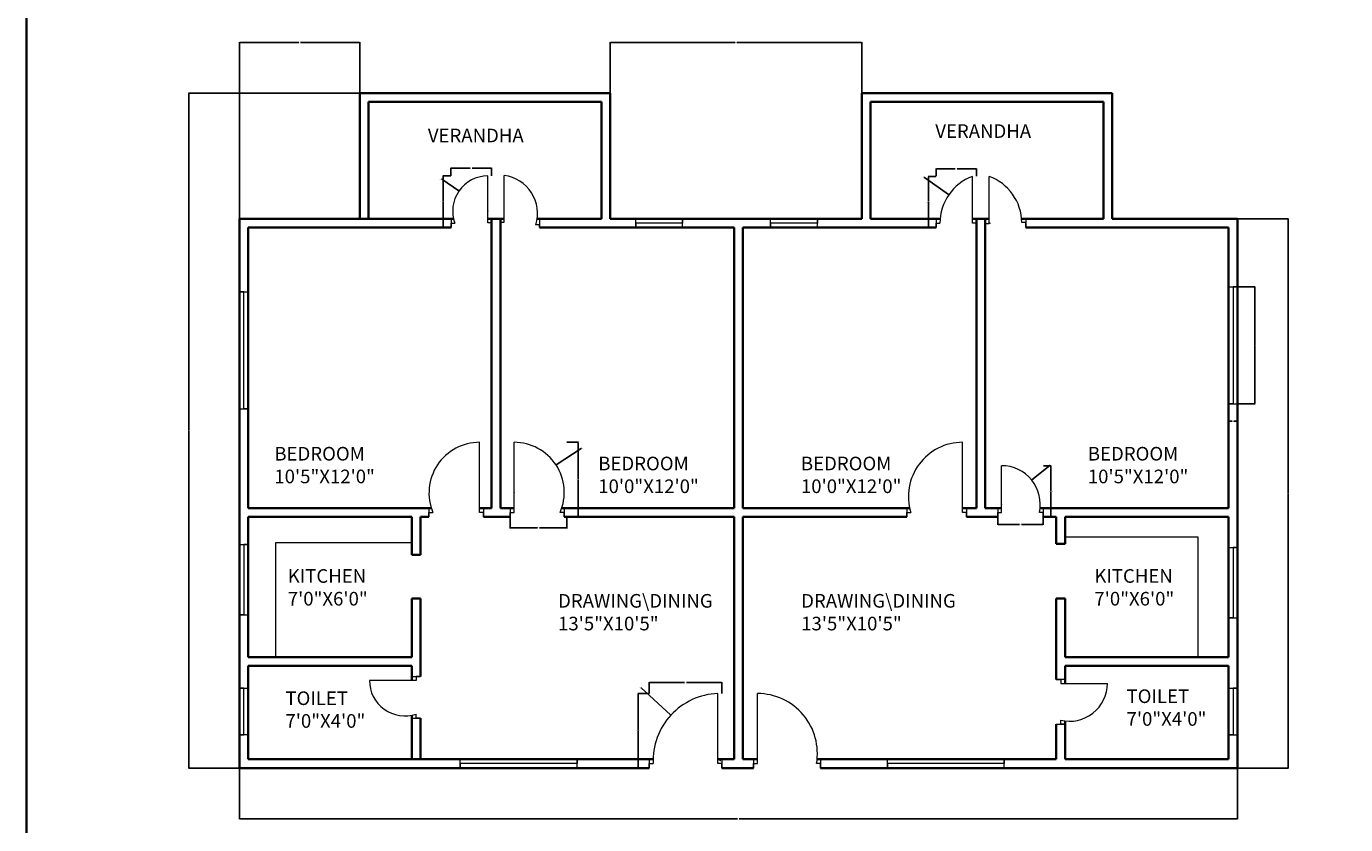
# Model space of a CAD drawing. Units: inches. Extents: x 2055 to 3558, y 1520 to 2888.
# Tile 3 of 8: x 2055 to 2732, y 2079 to 2489. Entities that reach past the tile are written whole.
import ezdxf

# ---------------------------------------------------------------- set-up
doc = ezdxf.new("R2010")
doc.units = ezdxf.units.IN
for name, color, linetype, lineweight in [('A-ANNO-DIMS', 2, 'Continuous', 18), ('A-ANNO-TTLB', 7, 'Continuous', 35), ('A-AREA-IDEN', 7, 'Continuous', 18), ('A-DOOR', 3, 'Continuous', 18), ('A-FLOR-FIXT', 8, 'Continuous', 18), ('A-GLAZ', 4, 'Continuous', 18), ('A-WALL', 7, 'Continuous', 35)]:
    doc.layers.add(name, color=color, linetype=linetype, lineweight=lineweight)
doc.styles.get("Standard").update_dxf_attribs({"font": 'arial.ttf'})
doc.dimstyles.get("Standard").update_dxf_attribs({"dimtxt": 0.18, "dimasz": 0.18, "dimexe": 0.18, "dimexo": 0.0625, "dimgap": 0.09, "dimtad": 0, "dimtih": 1, "dimtoh": 1, "dimdec": 4, "dimzin": 0, "dimdsep": 46, "dimtxsty": 'Standard', "dimcen": 0.09, "dimadec": 0, "dimazin": 0, "dimtfac": 1, "dimtdec": 4, "dimtofl": 0, "dimtmove": 0, "dimatfit": 3, "dimfxl": 1, "dimtolj": 1, "dimtzin": 0, "dimarcsym": 0})

# ---------------------------------------------------------------- blocks, each defined once
blk = doc.blocks.new('DOOR-BED-36-A')
for p, q in [((26, 2.25), (26, 38.25)), ((0, 4.5), (0, 0)), ((0, 0), (0, 2.25)), ((0, 2.25), (2, 2.25)), ((28, 2.25), (26, 2.25)), ((28, 4.5), (28, 0)), ((28, 0), (28, 2.25))]:
    blk.add_line(p, q)
blk.add_arc((26, 12.25), 26, 90, 202.62954)
blk = doc.blocks.new('DOOR-BED-36-B')
for p, q in [((2, 2.25), (2, 38.25)), ((0, 4.5), (0, 0)), ((0, 0), (0, 2.25)), ((0, 2.25), (2, 2.25)), ((27.66, 2.25), (25.66, 2.25)), ((27.66, 4.5), (27.66, 0)), ((27.66, 0), (27.66, 2.25))]:
    blk.add_line(p, q)
blk.add_arc((2, 12.47), 25.78, 336.6346, 90)
blk = doc.blocks.new('DOOR-BED-36-C')
for p, q in [((28.6, 2.25), (28.6, 38.25)), ((0, 4.5), (0, 0)), ((0, 0), (0, 2.25)), ((0, 2.25), (2, 2.25)), ((30.6, 2.25), (28.6, 2.25)), ((30.6, 4.5), (30.6, 0)), ((30.6, 0), (30.6, 2.25))]:
    blk.add_line(p, q)
blk.add_arc((28.6, 10.43), 27.83, 90, 197.08497)
blk = doc.blocks.new('DOOR-BED-24-A')
for p, q in [((2, 2.25), (2, 26.25)), ((0, 4.5), (0, 0)), ((0, 0), (0, 2.25)), ((0, 2.25), (2, 2.25)), ((23.39, 2.25), (21.39, 2.25)), ((23.39, 4.5), (23.39, 0)), ((23.39, 0), (23.39, 2.25))]:
    blk.add_line(p, q)
blk.add_arc((2, 6.42), 19.83, 347.8769, 90)
blk = doc.blocks.new('DOOR-BATH-24-A')
for p, q in [((4.5, 22.87), (0, 22.87)), ((0, 22.87), (2.25, 22.87)), ((2.25, 22.87), (2.25, 20.87)), ((2.25, 20.87), (26.25, 20.87)), ((2.25, 0), (2.25, 2)), ((0, 0), (4.5, 0)), ((4.5, 0), (2.25, 0))]:
    blk.add_line(p, q)
blk.add_arc((6.83, 20.87), 19.42, 256.35438, 0)
blk = doc.blocks.new('DOOR-ENTRY-36-A')
for p, q in [((2, 2.25), (2, 38.25)), ((0, 4.5), (0, 0)), ((0, 0), (0, 2.25)), ((0, 2.25), (2, 2.25)), ((34.35, 2.25), (32.35, 2.25)), ((34.35, 4.5), (34.35, 0)), ((34.35, 0), (34.35, 2.25))]:
    blk.add_line(p, q)
blk.add_arc((2, 7.46), 30.8, 350.26968, 90)
blk = doc.blocks.new('DOOR-ENTRY-36-B')
for p, q in [((35.2, 2.25), (35.2, 38.25)), ((0, 4.5), (0, 0)), ((0, 0), (0, 2.25)), ((0, 2.25), (2, 2.25)), ((37.2, 2.25), (35.2, 2.25)), ((37.2, 4.5), (37.2, 0)), ((37.2, 0), (37.2, 2.25))]:
    blk.add_line(p, q)
blk.add_arc((36.42, 3.82), 34.45, 92.03168, 182.60616)
blk = doc.blocks.new('DOOR-VERANDA-24-E')
for p, q in [((2, 2.71), (2, 26.71)), ((0, 2.71), (2, 2.71)), ((20.12, 1.44), (18.12, 1.44)), ((20.12, 4.5), (20.12, 0)), ((20.12, 0), (20.12, 1.44))]:
    blk.add_line(p, q)
blk.add_arc((-0.34, 7.44), 19.42, 342.01317, 83.06507)
blk = doc.blocks.new('DOOR-VERANDA-24-F')
for p, q in [((18.85, 2.51), (18.85, 26.51)), ((0, 4.5), (0, 0)), ((0, 0), (0, 2.25)), ((0, 2.25), (2, 2.25)), ((20.85, 2.51), (18.85, 2.51))]:
    blk.add_line(p, q)
blk.add_arc((18.85, 8.53), 17.98, 90, 200.4386)
blk = doc.blocks.new('DOOR-VERANDA-24-G')
for p, q in [((18.74, 2.29), (18.74, 26.29)), ((0, 4.5), (0, 0)), ((0, 0), (0, 2.25)), ((0, 2.25), (2, 2.25)), ((20.74, 2.29), (18.74, 2.29))]:
    blk.add_line(p, q)
blk.add_arc((27.63, 2.25), 25.63, 110.29699, 180)
blk = doc.blocks.new('DOOR-VERANDA-24-H')
for p, q in [((2, 2.19), (2, 26.19)), ((0, 2.19), (2, 2.19)), ((20.78, 2.69), (18.78, 2.69)), ((20.78, 4.5), (20.78, 0)), ((20.78, 0), (20.78, 2.69))]:
    blk.add_line(p, q)
blk.add_arc((-6.63, 2.38), 25.41, 0.68308, 70.14714)
blk = doc.blocks.new('DOOR-BATH-24-D')
for p, q in [((21.75, 21.33), (26.25, 21.33)), ((26.25, 21.33), (24, 21.33)), ((24, 21.33), (24, 19.33)), ((24, 19.33), (0, 19.33)), ((21.75, 0), (26.25, 0)), ((24, 0), (24, 2)), ((26.25, 0), (24, 0))]:
    blk.add_line(p, q)
blk.add_arc((18.26, 19.33), 18.26, 180, 288.33755)
blk = doc.blocks.new('WIN-36')
for p, q in [((2.25, 36), (0, 36)), ((0, 36), (4.5, 36)), ((2.25, 0), (2.25, 36)), ((0, 0), (4.5, 0)), ((4.5, 0), (2.25, 0))]:
    blk.add_line(p, q)
blk = doc.blocks.new('WIN-24')
for p, q in [((0, 24), (4.5, 24)), ((4.5, 24), (2.25, 24)), ((2.25, 24), (2.25, 0)), ((2.25, 0), (0, 0)), ((0, 0), (4.5, 0))]:
    blk.add_line(p, q)
blk = doc.blocks.new('WIN-24-2')
for p, q in [((2.25, 24), (0, 24)), ((0, 24), (4.5, 24)), ((2.25, 0), (2.25, 24)), ((4.5, 0), (0, 0)), ((0, 0), (2.25, 0))]:
    blk.add_line(p, q)
blk = doc.blocks.new('WIN-60')
for p, q in [((0, 60), (4.5, 60)), ((4.5, 60), (2.25, 60)), ((2.25, 60), (2.25, 0)), ((2.25, 0), (0, 0)), ((0, 0), (4.5, 0))]:
    blk.add_line(p, q)
blk = doc.blocks.new('COUNTER-1')
for p, q in [((70.02, 58.69), (0, 58.69)), ((0, 58.69), (0, 0))]:
    blk.add_line(p, q)
blk = doc.blocks.new('COUNTER-2')
for p, q in [((0, 61.79), (68.13, 61.79)), ((68.13, 61.79), (68.13, 0))]:
    blk.add_line(p, q)
blk = doc.blocks.new('VERANDA-PERIMETER')
for p, q in [((0, 0), (0, 64.5)), ((4.5, 64.5), (4.5, 4.5)), ((124.15, 4.5), (124.15, 64.5)), ((128.65, 64.5), (128.65, 4.5)), ((4.5, 0), (0, 0)), ((4.5, 4.5), (124.15, 4.5)), ((128.65, 0), (4.5, 0)), ((128.65, 4.5), (128.65, 0))]:
    blk.add_line(p, q)
blk = doc.blocks.new('*D44')
at = {"layer": 'A-ANNO-DIMS', "color": 0, "lineweight": -2, "transparency": 16777216}
for p, q in [((2676.74, 2355.07), (2685.85, 2355.07)), ((2685.67, 2354.89), (2685.67, 2325.25)), ((2685.67, 2295.25), (2685.67, 2324.88)), ((2676.74, 2295.07), (2685.85, 2295.07))]:
    blk.add_line(p, q, dxfattribs=at)
at = {"layer": 'A-ANNO-DIMS', "color": 0, "transparency": 16777216}
for points in [[(2685.64, 2354.89), (2685.7, 2354.89), (2685.67, 2355.07)], [(2685.64, 2295.25), (2685.7, 2295.25), (2685.67, 2295.07)]]:
    blk.add_solid(points, dxfattribs=at)
at = {"layer": 'Defpoints', "color": 0, "transparency": 16777216}
for p in [(2676.67, 2355.07), (2685.67, 2355.07), (2676.67, 2295.07)]:
    blk.add_point(p, dxfattribs=at)
at = {"layer": 'A-ANNO-DIMS', "color": 0, "transparency": 16777216, "insert": (2685.67, 2325.07), "char_height": 0.18, "attachment_point": 5}
blk.add_mtext('\\A1;WINDOW 60 TYP.', dxfattribs=at)
blk = doc.blocks.new('*D45')
at = {"layer": 'A-ANNO-DIMS', "color": 0, "lineweight": -2, "transparency": 16777216}
for p, q in [((2672.17, 2295), (2672.17, 2285.89)), ((2676.67, 2295), (2676.67, 2285.89)), ((2672.35, 2286.07), (2673.97, 2286.07)), ((2676.49, 2286.07), (2674.88, 2286.07))]:
    blk.add_line(p, q, dxfattribs=at)
at = {"layer": 'A-ANNO-DIMS', "color": 0, "transparency": 16777216}
for points in [[(2672.35, 2286.1), (2672.35, 2286.04), (2672.17, 2286.07)], [(2676.49, 2286.1), (2676.49, 2286.04), (2676.67, 2286.07)]]:
    blk.add_solid(points, dxfattribs=at)
at = {"layer": 'Defpoints', "color": 0, "transparency": 16777216}
for p in [(2672.17, 2295.07), (2676.67, 2295.07), (2676.67, 2286.07)]:
    blk.add_point(p, dxfattribs=at)
at = {"layer": 'A-ANNO-DIMS', "color": 0, "transparency": 16777216, "insert": (2674.42, 2286.07), "char_height": 0.18, "attachment_point": 5}
blk.add_mtext('\\A1;5 TYP.', dxfattribs=at)
blk = doc.blocks.new('*D54')
at = {"layer": 'A-ANNO-DIMS', "color": 0, "lineweight": -2, "transparency": 16777216}
for p, q in [((2332.38, 2275.25), (2338.24, 2275.25)), ((2338.06, 2275.07), (2338.06, 2256.31)), ((2338.06, 2237.18), (2338.06, 2255.94)), ((2332.38, 2237), (2338.24, 2237))]:
    blk.add_line(p, q, dxfattribs=at)
at = {"layer": 'A-ANNO-DIMS', "color": 0, "transparency": 16777216}
for points in [[(2338.03, 2275.07), (2338.09, 2275.07), (2338.06, 2275.25)], [(2338.03, 2237.18), (2338.09, 2237.18), (2338.06, 2237)]]:
    blk.add_solid(points, dxfattribs=at)
at = {"layer": 'Defpoints', "color": 0, "transparency": 16777216}
for p in [(2332.32, 2275.25), (2338.06, 2275.25), (2332.32, 2237)]:
    blk.add_point(p, dxfattribs=at)
at = {"layer": 'A-ANNO-DIMS', "color": 0, "transparency": 16777216, "insert": (2338.06, 2256.12), "char_height": 0.18, "attachment_point": 5}
blk.add_mtext('\\A1;BED DOOR 38 TYP.', dxfattribs=at)
blk = doc.blocks.new('*D55')
at = {"layer": 'A-ANNO-DIMS', "color": 0, "lineweight": -2, "transparency": 16777216}
for p, q in [((2303.21, 2236.94), (2303.21, 2231.08)), ((2332.32, 2236.94), (2332.32, 2231.08)), ((2303.39, 2231.26), (2317.24, 2231.26)), ((2332.14, 2231.26), (2318.3, 2231.26))]:
    blk.add_line(p, q, dxfattribs=at)
at = {"layer": 'A-ANNO-DIMS', "color": 0, "transparency": 16777216}
for points in [[(2303.39, 2231.29), (2303.39, 2231.23), (2303.21, 2231.26)], [(2332.14, 2231.29), (2332.14, 2231.23), (2332.32, 2231.26)]]:
    blk.add_solid(points, dxfattribs=at)
at = {"layer": 'Defpoints', "color": 0, "transparency": 16777216}
for p in [(2303.21, 2237), (2332.32, 2237), (2332.32, 2231.26)]:
    blk.add_point(p, dxfattribs=at)
at = {"layer": 'A-ANNO-DIMS', "color": 0, "transparency": 16777216, "insert": (2317.77, 2231.26), "char_height": 0.18, "attachment_point": 5}
blk.add_mtext('\\A1;29 TYP.', dxfattribs=at)
blk = doc.blocks.new('*D58')
at = {"layer": 'A-ANNO-DIMS', "color": 0, "lineweight": -2, "transparency": 16777216}
for p, q in [((2577.07, 2263.25), (2581.12, 2263.25)), ((2580.94, 2263.07), (2580.94, 2250.31)), ((2580.94, 2237.18), (2580.94, 2249.94)), ((2577.07, 2237), (2581.12, 2237))]:
    blk.add_line(p, q, dxfattribs=at)
at = {"layer": 'A-ANNO-DIMS', "color": 0, "transparency": 16777216}
for points in [[(2580.91, 2263.07), (2580.97, 2263.07), (2580.94, 2263.25)], [(2580.91, 2237.18), (2580.97, 2237.18), (2580.94, 2237)]]:
    blk.add_solid(points, dxfattribs=at)
at = {"layer": 'Defpoints', "color": 0, "transparency": 16777216}
for p in [(2577.01, 2263.25), (2580.94, 2263.25), (2577.01, 2237)]:
    blk.add_point(p, dxfattribs=at)
at = {"layer": 'A-ANNO-DIMS', "color": 0, "transparency": 16777216, "insert": (2580.94, 2250.12), "char_height": 0.18, "attachment_point": 5}
blk.add_mtext('\\A1;BED DOOR 26 TYP.', dxfattribs=at)
blk = doc.blocks.new('*D59')
at = {"layer": 'A-ANNO-DIMS', "color": 0, "lineweight": -2, "transparency": 16777216}
for p, q in [((2553.61, 2236.94), (2553.61, 2232.88)), ((2577.01, 2236.94), (2577.01, 2232.88)), ((2553.79, 2233.06), (2564.78, 2233.06)), ((2576.83, 2233.06), (2565.84, 2233.06))]:
    blk.add_line(p, q, dxfattribs=at)
at = {"layer": 'A-ANNO-DIMS', "color": 0, "transparency": 16777216}
for points in [[(2553.79, 2233.09), (2553.79, 2233.03), (2553.61, 2233.06)], [(2576.83, 2233.09), (2576.83, 2233.03), (2577.01, 2233.06)]]:
    blk.add_solid(points, dxfattribs=at)
at = {"layer": 'Defpoints', "color": 0, "transparency": 16777216}
for p in [(2553.61, 2237), (2577.01, 2237), (2577.01, 2233.06)]:
    blk.add_point(p, dxfattribs=at)
at = {"layer": 'A-ANNO-DIMS', "color": 0, "transparency": 16777216, "insert": (2565.31, 2233.06), "char_height": 0.18, "attachment_point": 5}
blk.add_mtext('\\A1;23 TYP.', dxfattribs=at)
blk = doc.blocks.new('*D64')
at = {"layer": 'A-ANNO-DIMS', "color": 0, "lineweight": -2, "transparency": 16777216}
for p, q in [((2374.6, 2146.25), (2368.74, 2146.25)), ((2368.92, 2146.07), (2368.92, 2127.31)), ((2368.92, 2108.18), (2368.92, 2126.94)), ((2374.6, 2108), (2368.74, 2108))]:
    blk.add_line(p, q, dxfattribs=at)
at = {"layer": 'A-ANNO-DIMS', "color": 0, "transparency": 16777216}
for points in [[(2368.89, 2146.07), (2368.95, 2146.07), (2368.92, 2146.25)], [(2368.89, 2108.18), (2368.95, 2108.18), (2368.92, 2108)]]:
    blk.add_solid(points, dxfattribs=at)
at = {"layer": 'Defpoints', "color": 0, "transparency": 16777216}
for p in [(2368.92, 2146.25), (2374.66, 2146.25), (2374.66, 2108)]:
    blk.add_point(p, dxfattribs=at)
at = {"layer": 'A-ANNO-DIMS', "color": 0, "transparency": 16777216, "insert": (2368.92, 2127.12), "char_height": 0.18, "attachment_point": 5}
blk.add_mtext('\\A1;ENTRY DOOR 38 TYP.', dxfattribs=at)
blk = doc.blocks.new('*D65')
at = {"layer": 'A-ANNO-DIMS', "color": 0, "lineweight": -2, "transparency": 16777216}
for p, q in [((2374.66, 2146.31), (2374.66, 2152.17)), ((2374.84, 2151.99), (2392.73, 2151.99)), ((2411.68, 2151.99), (2393.79, 2151.99)), ((2411.86, 2146.31), (2411.86, 2152.17))]:
    blk.add_line(p, q, dxfattribs=at)
at = {"layer": 'A-ANNO-DIMS', "color": 0, "transparency": 16777216}
for points in [[(2374.84, 2152.02), (2374.84, 2151.96), (2374.66, 2151.99)], [(2411.68, 2152.02), (2411.68, 2151.96), (2411.86, 2151.99)]]:
    blk.add_solid(points, dxfattribs=at)
at = {"layer": 'Defpoints', "color": 0, "transparency": 16777216}
for p in [(2411.86, 2151.99), (2374.66, 2146.25), (2411.86, 2146.25)]:
    blk.add_point(p, dxfattribs=at)
at = {"layer": 'A-ANNO-DIMS', "color": 0, "transparency": 16777216, "insert": (2393.26, 2151.99), "char_height": 0.18, "attachment_point": 5}
blk.add_mtext('\\A1;37 TYP.', dxfattribs=at)
blk = doc.blocks.new('*D92')
at = {"layer": 'A-ANNO-DIMS', "color": 0, "lineweight": -2, "transparency": 16777216}
for p, q in [((2272.7, 2412.01), (2268.61, 2412.01)), ((2268.79, 2411.83), (2268.79, 2398.94)), ((2268.79, 2385.68), (2268.79, 2398.57)), ((2272.7, 2385.5), (2268.61, 2385.5))]:
    blk.add_line(p, q, dxfattribs=at)
at = {"layer": 'A-ANNO-DIMS', "color": 0, "transparency": 16777216}
for points in [[(2268.76, 2411.83), (2268.82, 2411.83), (2268.79, 2412.01)], [(2268.76, 2385.68), (2268.82, 2385.68), (2268.79, 2385.5)]]:
    blk.add_solid(points, dxfattribs=at)
at = {"layer": 'Defpoints', "color": 0, "transparency": 16777216}
for p in [(2268.79, 2412.01), (2272.77, 2412.01), (2272.77, 2385.5)]:
    blk.add_point(p, dxfattribs=at)
at = {"layer": 'A-ANNO-DIMS', "color": 0, "transparency": 16777216, "insert": (2268.79, 2398.76), "char_height": 0.18, "attachment_point": 5}
blk.add_mtext('\\A1;VERANDA DOOR 27 TYP.', dxfattribs=at)
blk = doc.blocks.new('*D93')
at = {"layer": 'A-ANNO-DIMS', "color": 0, "lineweight": -2, "transparency": 16777216}
for p, q in [((2272.77, 2412.08), (2272.77, 2416.17)), ((2272.95, 2415.99), (2282.69, 2415.99)), ((2293.49, 2415.99), (2283.75, 2415.99)), ((2293.67, 2412.08), (2293.67, 2416.17))]:
    blk.add_line(p, q, dxfattribs=at)
at = {"layer": 'A-ANNO-DIMS', "color": 0, "transparency": 16777216}
for points in [[(2272.95, 2416.02), (2272.95, 2415.96), (2272.77, 2415.99)], [(2293.49, 2416.02), (2293.49, 2415.96), (2293.67, 2415.99)]]:
    blk.add_solid(points, dxfattribs=at)
at = {"layer": 'Defpoints', "color": 0, "transparency": 16777216}
for p in [(2272.77, 2412.01), (2293.67, 2415.99), (2293.67, 2412.01)]:
    blk.add_point(p, dxfattribs=at)
at = {"layer": 'A-ANNO-DIMS', "color": 0, "transparency": 16777216, "insert": (2283.22, 2415.99), "char_height": 0.18, "attachment_point": 5}
blk.add_mtext('\\A1;21 TYP.', dxfattribs=at)
blk = doc.blocks.new('*D94')
at = {"layer": 'A-ANNO-DIMS', "color": 0, "lineweight": -2, "transparency": 16777216}
for p, q in [((2521.87, 2411.79), (2517.81, 2411.79)), ((2517.99, 2411.61), (2517.99, 2398.83)), ((2517.99, 2385.68), (2517.99, 2398.46)), ((2521.87, 2385.5), (2517.81, 2385.5))]:
    blk.add_line(p, q, dxfattribs=at)
at = {"layer": 'A-ANNO-DIMS', "color": 0, "transparency": 16777216}
for points in [[(2517.96, 2411.61), (2518.02, 2411.61), (2517.99, 2411.79)], [(2517.96, 2385.68), (2518.02, 2385.68), (2517.99, 2385.5)]]:
    blk.add_solid(points, dxfattribs=at)
at = {"layer": 'Defpoints', "color": 0, "transparency": 16777216}
for p in [(2517.99, 2411.79), (2521.94, 2411.79), (2521.94, 2385.5)]:
    blk.add_point(p, dxfattribs=at)
at = {"layer": 'A-ANNO-DIMS', "color": 0, "transparency": 16777216, "insert": (2517.99, 2398.64), "char_height": 0.18, "attachment_point": 5}
blk.add_mtext('\\A1;VERANDA DOOR 26 TYP.', dxfattribs=at)
blk = doc.blocks.new('*D95')
at = {"layer": 'A-ANNO-DIMS', "color": 0, "lineweight": -2, "transparency": 16777216}
for p, q in [((2521.94, 2411.85), (2521.94, 2415.91)), ((2522.12, 2415.73), (2531.78, 2415.73)), ((2542.49, 2415.73), (2532.84, 2415.73)), ((2542.67, 2411.85), (2542.67, 2415.91))]:
    blk.add_line(p, q, dxfattribs=at)
at = {"layer": 'A-ANNO-DIMS', "color": 0, "transparency": 16777216}
for points in [[(2522.12, 2415.76), (2522.12, 2415.7), (2521.94, 2415.73)], [(2542.49, 2415.76), (2542.49, 2415.7), (2542.67, 2415.73)]]:
    blk.add_solid(points, dxfattribs=at)
at = {"layer": 'Defpoints', "color": 0, "transparency": 16777216}
for p in [(2542.67, 2415.73), (2521.94, 2411.79), (2542.67, 2411.79)]:
    blk.add_point(p, dxfattribs=at)
at = {"layer": 'A-ANNO-DIMS', "color": 0, "transparency": 16777216, "insert": (2532.31, 2415.73), "char_height": 0.18, "attachment_point": 5}
blk.add_mtext('\\A1;21 TYP.', dxfattribs=at)
blk = doc.blocks.new('*D118')
at = {"layer": 'A-ANNO-DIMS', "color": 0, "lineweight": -2, "transparency": 16777216}
for p, q in [((2164.17, 2107.94), (2164.17, 2081.77)), ((2676.67, 2107.94), (2676.67, 2081.77)), ((2164.35, 2081.95), (2420.03, 2081.95)), ((2676.49, 2081.95), (2420.82, 2081.95))]:
    blk.add_line(p, q, dxfattribs=at)
at = {"layer": 'A-ANNO-DIMS', "color": 0, "transparency": 16777216}
for points in [[(2164.35, 2081.98), (2164.35, 2081.92), (2164.17, 2081.95)], [(2676.49, 2081.98), (2676.49, 2081.92), (2676.67, 2081.95)]]:
    blk.add_solid(points, dxfattribs=at)
at = {"layer": 'Defpoints', "color": 0, "transparency": 16777216}
for p in [(2164.17, 2108), (2676.67, 2108), (2676.67, 2081.95)]:
    blk.add_point(p, dxfattribs=at)
at = {"layer": 'A-ANNO-DIMS', "color": 0, "transparency": 16777216, "insert": (2420.42, 2081.95), "char_height": 0.18, "attachment_point": 5}
blk.add_mtext('\\A1;512.5', dxfattribs=at)
blk = doc.blocks.new('*D119')
at = {"layer": 'A-ANNO-DIMS', "color": 0, "lineweight": -2, "transparency": 16777216}
for p, q in [((2225.88, 2454.5), (2137.94, 2454.5)), ((2138.12, 2454.32), (2138.12, 2281.43)), ((2138.12, 2108.18), (2138.12, 2281.07)), ((2164.11, 2108), (2137.94, 2108))]:
    blk.add_line(p, q, dxfattribs=at)
at = {"layer": 'A-ANNO-DIMS', "color": 0, "transparency": 16777216}
for points in [[(2138.09, 2454.32), (2138.15, 2454.32), (2138.12, 2454.5)], [(2138.09, 2108.18), (2138.15, 2108.18), (2138.12, 2108)]]:
    blk.add_solid(points, dxfattribs=at)
at = {"layer": 'Defpoints', "color": 0, "transparency": 16777216}
for p in [(2138.12, 2454.5), (2225.95, 2454.5), (2164.17, 2108)]:
    blk.add_point(p, dxfattribs=at)
at = {"layer": 'A-ANNO-DIMS', "color": 0, "transparency": 16777216, "insert": (2138.12, 2281.25), "char_height": 0.18, "attachment_point": 5}
blk.add_mtext('\\A1;346.5', dxfattribs=at)
blk = doc.blocks.new('*D120')
at = {"layer": 'A-ANNO-DIMS', "color": 0, "lineweight": -2, "transparency": 16777216}
for p, q in [((2676.74, 2390), (2702.9, 2390)), ((2702.72, 2389.82), (2702.72, 2249.18)), ((2702.72, 2108.18), (2702.72, 2248.82)), ((2676.74, 2108), (2702.9, 2108))]:
    blk.add_line(p, q, dxfattribs=at)
at = {"layer": 'A-ANNO-DIMS', "color": 0, "transparency": 16777216}
for points in [[(2702.69, 2389.82), (2702.75, 2389.82), (2702.72, 2390)], [(2702.69, 2108.18), (2702.75, 2108.18), (2702.72, 2108)]]:
    blk.add_solid(points, dxfattribs=at)
at = {"layer": 'Defpoints', "color": 0, "transparency": 16777216}
for p in [(2676.67, 2390), (2702.72, 2390), (2676.67, 2108)]:
    blk.add_point(p, dxfattribs=at)
at = {"layer": 'A-ANNO-DIMS', "color": 0, "transparency": 16777216, "insert": (2702.72, 2249), "char_height": 0.18, "attachment_point": 5}
blk.add_mtext('\\A1;282', dxfattribs=at)
blk = doc.blocks.new('*D126')
at = {"layer": 'A-ANNO-DIMS', "color": 0, "lineweight": -2, "transparency": 16777216}
for p, q in [((2164.17, 2390.06), (2164.17, 2480.73)), ((2164.35, 2480.55), (2194.67, 2480.55)), ((2225.77, 2480.55), (2195.45, 2480.55)), ((2225.95, 2390.06), (2225.95, 2480.73))]:
    blk.add_line(p, q, dxfattribs=at)
at = {"layer": 'A-ANNO-DIMS', "color": 0, "transparency": 16777216}
for points in [[(2164.35, 2480.58), (2164.35, 2480.52), (2164.17, 2480.55)], [(2225.77, 2480.58), (2225.77, 2480.52), (2225.95, 2480.55)]]:
    blk.add_solid(points, dxfattribs=at)
at = {"layer": 'Defpoints', "color": 0, "transparency": 16777216}
for p in [(2225.95, 2480.55), (2164.17, 2390), (2225.95, 2390)]:
    blk.add_point(p, dxfattribs=at)
at = {"layer": 'A-ANNO-DIMS', "color": 0, "transparency": 16777216, "insert": (2195.06, 2480.55), "char_height": 0.18, "attachment_point": 5}
blk.add_mtext('\\A1;61.77', dxfattribs=at)
blk = doc.blocks.new('*D127')
at = {"layer": 'A-ANNO-DIMS', "color": 0, "lineweight": -2, "transparency": 16777216}
for p, q in [((2354.59, 2454.56), (2354.59, 2480.73)), ((2354.77, 2480.55), (2418.72, 2480.55)), ((2483.58, 2480.55), (2419.63, 2480.55)), ((2483.76, 2454.56), (2483.76, 2480.73))]:
    blk.add_line(p, q, dxfattribs=at)
at = {"layer": 'A-ANNO-DIMS', "color": 0, "transparency": 16777216}
for points in [[(2354.77, 2480.58), (2354.77, 2480.52), (2354.59, 2480.55)], [(2483.58, 2480.58), (2483.58, 2480.52), (2483.76, 2480.55)]]:
    blk.add_solid(points, dxfattribs=at)
at = {"layer": 'Defpoints', "color": 0, "transparency": 16777216}
for p in [(2483.76, 2480.55), (2354.59, 2454.5), (2483.76, 2454.5)]:
    blk.add_point(p, dxfattribs=at)
at = {"layer": 'A-ANNO-DIMS', "color": 0, "transparency": 16777216, "insert": (2419.17, 2480.55), "char_height": 0.18, "attachment_point": 5}
blk.add_mtext('\\A1;129.16', dxfattribs=at)
blk = doc.blocks.new('*D161')
at = {"layer": 'A-ANNO-DIMS', "color": 0, "lineweight": -2, "transparency": 16777216}
for p, q in [((2370.37, 2149.19), (2370.55, 2149.19)), ((2370.55, 2149.19), (2385.62, 2135.3)), ((2410.99, 2111.82), (2411.17, 2111.82)), ((2411.08, 2111.73), (2411.08, 2111.91))]:
    blk.add_line(p, q, dxfattribs=at)
at = {"layer": 'A-ANNO-DIMS', "color": 0, "transparency": 16777216}
blk.add_solid([(2385.64, 2135.32), (2385.6, 2135.27), (2385.75, 2135.17)], dxfattribs=at)
at = {"layer": 'Defpoints', "color": 0, "transparency": 16777216}
for p in [(2385.75, 2135.17), (2411.08, 2111.82)]:
    blk.add_point(p, dxfattribs=at)
at = {"layer": 'A-ANNO-DIMS', "color": 0, "transparency": 16777216, "insert": (2369.82, 2149.19), "char_height": 0.18, "attachment_point": 5}
blk.add_mtext('\\A1;R34.455', dxfattribs=at)
blk = doc.blocks.new('*D165')
at = {"layer": 'A-ANNO-DIMS', "color": 0, "lineweight": -2, "transparency": 16777216}
for p, q in [((2339.68, 2272.13), (2326.9, 2263.73)), ((2339.86, 2272.13), (2339.68, 2272.13)), ((2305.12, 2249.47), (2305.3, 2249.47)), ((2305.21, 2249.38), (2305.21, 2249.56))]:
    blk.add_line(p, q, dxfattribs=at)
at = {"layer": 'A-ANNO-DIMS', "color": 0, "transparency": 16777216}
blk.add_solid([(2326.89, 2263.75), (2326.92, 2263.7), (2326.75, 2263.63)], dxfattribs=at)
at = {"layer": 'Defpoints', "color": 0, "transparency": 16777216}
for p in [(2326.75, 2263.63), (2305.21, 2249.47)]:
    blk.add_point(p, dxfattribs=at)
at = {"layer": 'A-ANNO-DIMS', "color": 0, "transparency": 16777216, "insert": (2340.41, 2272.13), "char_height": 0.18, "attachment_point": 5}
blk.add_mtext('\\A1;R25.777', dxfattribs=at)
blk = doc.blocks.new('*D166')
at = {"layer": 'A-ANNO-DIMS', "color": 0, "lineweight": -2, "transparency": 16777216}
for p, q in [((2515.73, 2411.18), (2515.91, 2411.18)), ((2515.91, 2411.18), (2528.39, 2402.5)), ((2549.47, 2387.75), (2549.65, 2387.75)), ((2549.56, 2387.66), (2549.56, 2387.84))]:
    blk.add_line(p, q, dxfattribs=at)
at = {"layer": 'A-ANNO-DIMS', "color": 0, "transparency": 16777216}
blk.add_solid([(2528.4, 2402.52), (2528.37, 2402.47), (2528.53, 2402.39)], dxfattribs=at)
at = {"layer": 'Defpoints', "color": 0, "transparency": 16777216}
for p in [(2528.53, 2402.39), (2549.56, 2387.75)]:
    blk.add_point(p, dxfattribs=at)
at = {"layer": 'A-ANNO-DIMS', "color": 0, "transparency": 16777216, "insert": (2515.25, 2411.18), "char_height": 0.18, "attachment_point": 5}
blk.add_mtext('\\A1;R25.63', dxfattribs=at)
blk = doc.blocks.new('*D168')
at = {"layer": 'A-ANNO-DIMS', "color": 0, "lineweight": -2, "transparency": 16777216}
for p, q in [((2580.3, 2263.36), (2571.18, 2255.99)), ((2580.48, 2263.36), (2580.3, 2263.36)), ((2555.52, 2243.41), (2555.7, 2243.41)), ((2555.61, 2243.32), (2555.61, 2243.5))]:
    blk.add_line(p, q, dxfattribs=at)
at = {"layer": 'A-ANNO-DIMS', "color": 0, "transparency": 16777216}
blk.add_solid([(2571.16, 2256.02), (2571.2, 2255.97), (2571.04, 2255.88)], dxfattribs=at)
at = {"layer": 'Defpoints', "color": 0, "transparency": 16777216}
for p in [(2571.04, 2255.88), (2555.61, 2243.41)]:
    blk.add_point(p, dxfattribs=at)
at = {"layer": 'A-ANNO-DIMS', "color": 0, "transparency": 16777216, "insert": (2581.03, 2263.36), "char_height": 0.18, "attachment_point": 5}
blk.add_mtext('\\A1;R19.835', dxfattribs=at)
blk = doc.blocks.new('*D172')
at = {"layer": 'A-ANNO-DIMS', "color": 0, "lineweight": -2, "transparency": 16777216}
for p, q in [((2267.86, 2410.44), (2268.04, 2410.44)), ((2268.04, 2410.44), (2276.76, 2404.39)), ((2291.58, 2394.03), (2291.76, 2394.03)), ((2291.67, 2393.94), (2291.67, 2394.12))]:
    blk.add_line(p, q, dxfattribs=at)
at = {"layer": 'A-ANNO-DIMS', "color": 0, "transparency": 16777216}
blk.add_solid([(2276.77, 2404.42), (2276.74, 2404.37), (2276.9, 2404.29)], dxfattribs=at)
at = {"layer": 'Defpoints', "color": 0, "transparency": 16777216}
for p in [(2276.9, 2404.29), (2291.67, 2394.03)]:
    blk.add_point(p, dxfattribs=at)
at = {"layer": 'A-ANNO-DIMS', "color": 0, "transparency": 16777216, "insert": (2267.31, 2410.44), "char_height": 0.18, "attachment_point": 5}
blk.add_mtext('\\A1;R17.983', dxfattribs=at)

msp = doc.modelspace()

# ---------------------------------------------------------------- linework, layer by layer
at = {"layer": 'A-ANNO-TTLB'}
msp.add_lwpolyline([(2054.7598, 2888.2545), (3557.8479, 2888.2545), (3557.8479, 1520.3256), (2054.7598, 1520.3256)], close=True, dxfattribs=at)
at = {"layer": 'A-WALL'}
for p, q in [((2164.1747, 2389.9995), (2274.1485, 2389.9995)), ((2164.1747, 2389.9995), (2225.9468, 2389.9995)), ((2164.1747, 2389.9995), (2164.1747, 2107.9995)), ((2168.6747, 2385.4995), (2272.8233, 2385.4995)), ((2168.6747, 2385.4995), (2168.6747, 2241.4995)), ((2230.4468, 2389.9995), (2274.1485, 2389.9995)), ((2291.6747, 2389.9995), (2300.1747, 2389.9995)), ((2291.6747, 2389.9995), (2300.1747, 2389.9995)), ((2293.6747, 2389.9995), (2293.6747, 2241.4995)), ((2298.1747, 2389.9995), (2298.1747, 2241.4995)), ((2317.024, 2389.9995), (2350.0929, 2389.9995)), ((2317.024, 2389.9995), (2350.0929, 2389.9995)), ((2318.2986, 2385.4995), (2418.1747, 2385.4995)), ((2354.5929, 2389.9995), (2483.7569, 2389.9995)), ((2354.5929, 2389.9995), (2483.7569, 2389.9995)), ((2418.1747, 2385.4995), (2418.1747, 2241.4995)), ((2422.6747, 2385.4995), (2422.6747, 2241.4995)), ((2422.6747, 2385.4995), (2521.9367, 2385.4995)), ((2488.2569, 2389.9995), (2524.0357, 2389.9995)), ((2488.2569, 2389.9995), (2524.0357, 2389.9995)), ((2540.6747, 2389.9995), (2549.1747, 2389.9995)), ((2540.6747, 2389.9995), (2549.1747, 2389.9995)), ((2542.6747, 2389.9995), (2542.6747, 2241.4995)), ((2547.1747, 2389.9995), (2547.1747, 2241.4995)), ((2565.8698, 2389.9995), (2607.9031, 2389.9995)), ((2565.8698, 2389.9995), (2607.9031, 2389.9995)), ((2567.9564, 2385.4995), (2672.1747, 2385.4995)), ((2612.4031, 2389.9995), (2676.6747, 2389.9995)), ((2612.4031, 2389.9995), (2676.6747, 2389.9995)), ((2672.1747, 2385.4995), (2672.1747, 2241.4995)), ((2676.6747, 2389.9995), (2676.6747, 2107.9995)), ((2168.6747, 2241.4995), (2262.699, 2241.4995)), ((2168.6747, 2236.9995), (2252.6747, 2236.9995)), ((2168.6747, 2236.9995), (2168.6747, 2164.9995)), ((2252.6747, 2241.4995), (2257.1747, 2241.4995)), ((2252.6747, 2217.4337), (2252.6747, 2236.9995)), ((2257.1747, 2236.9995), (2257.1747, 2217.4337)), ((2257.1747, 2236.9995), (2261.5175, 2236.9995)), ((2287.5131, 2241.4995), (2293.6747, 2241.4995)), ((2289.5131, 2236.9995), (2303.2136, 2236.9995)), ((2298.1747, 2241.4995), (2305.2136, 2241.4995)), ((2329.7266, 2241.4995), (2418.1747, 2241.4995)), ((2330.8768, 2236.9995), (2418.1747, 2236.9995)), ((2418.1747, 2236.9995), (2418.1747, 2112.4995)), ((2422.6747, 2241.4995), (2508.3924, 2241.4995)), ((2422.6747, 2236.9995), (2422.6747, 2112.4995)), ((2422.6747, 2236.9995), (2506.9822, 2236.9995)), ((2535.5795, 2241.4995), (2542.6747, 2241.4995)), ((2537.5795, 2236.9995), (2553.6132, 2236.9995)), ((2547.1747, 2241.4995), (2555.6132, 2241.4995)), ((2575.355, 2241.4995), (2672.1747, 2241.4995)), ((2577.0054, 2236.9995), (2583.6747, 2236.9995)), ((2588.1747, 2241.4995), (2583.6747, 2241.4995)), ((2583.6747, 2236.9995), (2583.6747, 2223.192)), ((2588.1747, 2236.9995), (2672.1747, 2236.9995)), ((2588.1747, 2223.192), (2588.1747, 2236.9995)), ((2672.1747, 2236.9995), (2672.1747, 2164.9995)), ((2583.6747, 2223.192), (2588.1747, 2223.192)), ((2252.6747, 2217.4337), (2257.1747, 2217.4337)), ((2252.6747, 2164.9995), (2252.6747, 2194.987)), ((2252.6747, 2194.987), (2257.1747, 2194.987)), ((2257.1747, 2194.987), (2257.1747, 2155.0034)), ((2588.1747, 2194.9685), (2583.6747, 2194.9685)), ((2583.6747, 2194.9685), (2583.6747, 2153.4523)), ((2588.1747, 2164.9995), (2588.1747, 2194.9685)), ((2168.6747, 2164.9995), (2252.6747, 2164.9995)), ((2588.1747, 2164.9995), (2672.1747, 2164.9995)), ((2168.6747, 2160.4995), (2252.6747, 2160.4995)), ((2168.6747, 2160.4995), (2168.6747, 2112.4995)), ((2252.6747, 2153.0034), (2252.6747, 2160.4995)), ((2588.1747, 2160.4995), (2672.1747, 2160.4995)), ((2588.1747, 2151.4523), (2588.1747, 2160.4995)), ((2672.1747, 2160.4995), (2672.1747, 2112.4995)), ((2252.6747, 2112.4995), (2252.6747, 2135.0845)), ((2257.1747, 2133.6742), (2257.1747, 2112.4995)), ((2583.6747, 2130.5817), (2583.6747, 2112.4995)), ((2588.1747, 2112.4995), (2588.1747, 2132.174)), ((2164.1747, 2107.9995), (2374.6605, 2107.9995)), ((2164.1747, 2107.9995), (2374.6605, 2107.9995)), ((2168.6747, 2112.4995), (2376.6316, 2112.4995)), ((2168.6747, 2112.4995), (2252.6747, 2112.4995)), ((2409.8583, 2112.4995), (2418.1747, 2112.4995)), ((2411.8583, 2107.9995), (2428.1891, 2107.9995)), ((2411.8583, 2107.9995), (2418.1747, 2107.9995)), ((2422.6747, 2112.4995), (2430.1891, 2112.4995)), ((2460.8422, 2112.4995), (2583.6747, 2112.4995)), ((2462.5413, 2107.9995), (2676.6747, 2107.9995)), ((2588.1747, 2112.4995), (2672.1747, 2112.4995)), ((2672.1747, 2107.9995), (2588.1747, 2107.9995))]:
    msp.add_line(p, q, dxfattribs=at)

# ---------------------------------------------------------------- block references
at = {"layer": 'A-DOOR'}
for name, p in [('DOOR-VERANDA-24-F', (2272.823, 2385.499)), ('DOOR-VERANDA-24-E', (2298.175, 2385.499)), ('DOOR-VERANDA-24-G', (2521.937, 2385.499)), ('DOOR-VERANDA-24-H', (2547.175, 2385.499)), ('DOOR-BED-36-A', (2261.516, 2236.999)), ('DOOR-BED-36-B', (2303.214, 2236.999)), ('DOOR-BED-36-C', (2506.982, 2236.999)), ('DOOR-BED-24-A', (2553.613, 2236.999)), ('DOOR-BATH-24-D', (2230.925, 2133.674)), ('DOOR-BATH-24-A', (2583.675, 2130.582)), ('DOOR-ENTRY-36-B', (2374.66, 2107.999)), ('DOOR-ENTRY-36-A', (2428.189, 2107.999))]:
    msp.add_blockref(name, p, dxfattribs=at)
at = {"layer": 'A-FLOR-FIXT'}
for name, p in [('COUNTER-1', (2182.656, 2164.999)), ('COUNTER-2', (2588.175, 2164.999))]:
    msp.add_blockref(name, p, dxfattribs=at)
at = {"layer": 'A-GLAZ', "extrusion": (0, 0, -1), "zscale": -1}
for name, p, rotation in [('WIN-24', (-2367.7658, 2385.4998), 90), ('WIN-24', (-2436.9607, 2385.4998), 90), ('WIN-60', (-2164.175, 2352.516), 180), ('WIN-36', (-2164.175, 2222.7217), 180), ('WIN-36', (-2672.175, 2221.1923), 180), ('WIN-60', (-2277.5799, 2107.9998), 90), ('WIN-60', (-2496.9178, 2107.9998), 90)]:
    msp.add_blockref(name, p, dxfattribs=dict(at, rotation=rotation))
at = {"layer": 'A-GLAZ'}
for name, p in [('WIN-60', (2672.175, 2295.066)), ('WIN-24-2', (2164.175, 2124.998)), ('WIN-24', (2672.175, 2125.0333))]:
    msp.add_blockref(name, p, dxfattribs=at)
at = {"layer": 'A-WALL', "extrusion": (0, 0, -1), "zscale": -1, "rotation": 180}
for p in [(-2225.9468, 2454.5), (-2483.7569, 2454.5)]:
    msp.add_blockref('VERANDA-PERIMETER', p, dxfattribs=at)

# ---------------------------------------------------------------- texts
at = {"layer": 'A-AREA-IDEN', "char_height": 7, "attachment_point": 1}
for s, width, insert in [('VERANDHA', 73.975505, (2260.942, 2436.3006)), ('VERANDHA', 73.975505, (2521.528, 2438.5446)), ('BEDROOM\\P10\'5"X12\'0"', 285.522885, (2182.0987, 2272.8947)), ('BEDROOM\\P10\'5"X12\'0"', 285.522885, (2599.8629, 2272.8947)), ('BEDROOM\\P10\'0"X12\'0"', 113.389445, (2348.4409, 2267.8696)), ('BEDROOM\\P10\'0"X12\'0"', 113.389445, (2452.5191, 2267.8696)), ('KITCHEN\\P7\'0"X6\'0"', 92.673757, (2189.003, 2210.116)), ('KITCHEN\\P7\'0"X6\'0"', 92.673757, (2603.2271, 2210.116)), ('DRAWING\\\\DINING\\P13\'5"X10\'5"', 76.318653, (2327.8069, 2197.357)), ('DRAWING\\\\DINING\\P13\'5"X10\'5"', 76.318653, (2452.6588, 2197.357)), ('TOILET\\P7\'0"X4\'0"', 58.820839, (2619.7527, 2148.3795)), ('TOILET\\P7\'0"X4\'0"', 58.820839, (2187.7928, 2147.3458))]:
    msp.add_mtext_dynamic_manual_height_columns(s, width=width, gutter_width=12.5, heights=[0], dxfattribs=dict(at, insert=insert))

# ---------------------------------------------------------------- dimensions: what is measured, and where the dimension line sits
at = {"layer": 'A-ANNO-DIMS'}
for base, p1, p2, override, picture, middle in [((2225.9468, 2480.5495), (2164.1747, 2389.9995), (2225.9468, 2389.9995), {"dimdec": 2, "dimlfac": 1, "dimrnd": 0, "dimzin": 0, "dimdsep": 46, "dimlunit": 2}, '*D126', (2195.0607, 2480.5495)), ((2483.7569, 2480.5495), (2354.5929, 2454.4995), (2483.7569, 2454.4995), {"dimdec": 2, "dimlfac": 1, "dimrnd": 0, "dimzin": 0, "dimdsep": 46, "dimlunit": 2}, '*D127', (2419.1749, 2480.5495)), ((2676.6747, 2081.9495), (2164.1747, 2107.9995), (2676.6747, 2107.9995), {"dimdec": 1, "dimlfac": 1, "dimrnd": 0, "dimzin": 0, "dimdsep": 46, "dimlunit": 2}, '*D118', (2420.4247, 2081.9495))]:
    dim = msp.add_linear_dim(base=base, p1=p1, p2=p2, dimstyle='Standard', override=override, dxfattribs=at)
    dim.commit()
    dim.dimension.update_dxf_attribs({"geometry": picture, "text_midpoint": middle})
for base, p1, p2, override, picture, middle in [((2138.1247, 2454.4995), (2164.1747, 2107.9995), (2225.9468, 2454.4995), {"dimdec": 1, "dimlfac": 1, "dimrnd": 0, "dimzin": 0, "dimdsep": 46, "dimlunit": 2}, '*D119', (2138.1247, 2281.2495)), ((2702.7247, 2389.9995), (2676.6747, 2107.9995), (2676.6747, 2389.9995), {"dimdec": 0, "dimlfac": 1, "dimrnd": 0, "dimzin": 0, "dimdsep": 46, "dimlunit": 2}, '*D120', (2702.7247, 2248.9995))]:
    dim = msp.add_linear_dim(base=base, p1=p1, p2=p2, angle=90, dimstyle='Standard', override=override, dxfattribs=at)
    dim.commit()
    dim.dimension.update_dxf_attribs({"geometry": picture, "text_midpoint": middle})
for base, p1, p2, text, picture, middle in [((2268.7889, 2412.0129), (2272.7659, 2385.4995), (2272.7659, 2412.0129), 'VERANDA DOOR <> TYP.', '*D92', (2268.7889, 2398.7562)), ((2517.9937, 2411.7861), (2521.9367, 2385.4995), (2521.9367, 2411.7861), 'VERANDA DOOR <> TYP.', '*D94', (2517.9937, 2398.6428)), ((2685.6747, 2355.0661), (2676.6747, 2295.0661), (2676.6747, 2355.0661), 'WINDOW <> TYP.', '*D44', (2685.6747, 2325.0661)), ((2338.0559, 2275.2495), (2332.3184, 2236.9995), (2332.3184, 2275.2495), 'BED DOOR <> TYP.', '*D54', (2338.0559, 2256.1245)), ((2580.9429, 2263.2495), (2577.0054, 2236.9995), (2577.0054, 2263.2495), 'BED DOOR <> TYP.', '*D58', (2580.9429, 2250.1245)), ((2368.923, 2146.2495), (2374.6605, 2107.9995), (2374.6605, 2146.2495), 'ENTRY DOOR <> TYP.', '*D64', (2368.923, 2127.1245))]:
    dim = msp.add_linear_dim(base=base, p1=p1, p2=p2, angle=90, text=text, dimstyle='Standard', override={"dimdec": 0, "dimlfac": 1, "dimrnd": 0, "dimzin": 0, "dimdsep": 46, "dimlunit": 2}, dxfattribs=at)
    dim.commit()
    dim.dimension.update_dxf_attribs({"geometry": picture, "text_midpoint": middle})
for base, p1, p2, picture, middle in [((2293.6747, 2415.9899), (2272.7659, 2412.0129), (2293.6747, 2412.0129), '*D93', (2283.2203, 2415.9899)), ((2542.6747, 2415.7291), (2521.9367, 2411.7861), (2542.6747, 2411.7861), '*D95', (2532.3057, 2415.7291)), ((2676.6746671216, 2286.0661256488), (2672.1746671216, 2295.0661256488), (2676.6746671216, 2295.0661256488), '*D45', (2674.4246671216, 2286.0661256488)), ((2332.3184, 2231.262), (2303.2136, 2236.9995), (2332.3184, 2236.9995), '*D55', (2317.766, 2231.262)), ((2577.0054, 2233.062), (2553.6132, 2236.9995), (2577.0054, 2236.9995), '*D59', (2565.3093, 2233.062)), ((2411.8583, 2151.987), (2374.6605, 2146.2495), (2411.8583, 2146.2495), '*D65', (2393.2594, 2151.987))]:
    dim = msp.add_linear_dim(base=base, p1=p1, p2=p2, text='<> TYP.', dimstyle='Standard', override={"dimdec": 0, "dimlfac": 1, "dimrnd": 0, "dimzin": 0, "dimdsep": 46, "dimlunit": 2}, dxfattribs=at)
    dim.commit()
    dim.dimension.update_dxf_attribs({"geometry": picture, "text_midpoint": middle})
for center, mpoint, override, picture, middle in [((2291.67467, 2394.02939), (2276.90415, 2404.2879), {"dimdec": 3, "dimlfac": 1, "dimrnd": 0, "dimzin": 0, "dimdsep": 46, "dimlunit": 2}, '*D172', (2267.31208, 2410.443)), ((2549.5646, 2387.7495), (2528.5335, 2402.3947), {"dimdec": 2, "dimlfac": 1, "dimrnd": 0, "dimzin": 0, "dimdsep": 46, "dimlunit": 2}, '*D166', (2515.255, 2411.1818)), ((2305.2136, 2249.4725), (2326.7541, 2263.631), {"dimdec": 3, "dimlfac": 1, "dimrnd": 0, "dimzin": 0, "dimdsep": 46, "dimlunit": 2}, '*D165', (2340.4081, 2272.1262)), ((2555.61322, 2243.415), (2571.0408, 2255.88084), {"dimdec": 3, "dimlfac": 1, "dimrnd": 0, "dimzin": 0, "dimdsep": 46, "dimlunit": 2}, '*D168', (2581.02779, 2263.36034)), ((2411.0798, 2111.8162), (2385.7509, 2135.1741), {"dimdec": 3, "dimlfac": 1, "dimrnd": 0, "dimzin": 0, "dimdsep": 46, "dimlunit": 2}, '*D161', (2369.8231, 2149.1888))]:
    dim = msp.add_radius_dim(center=center, mpoint=mpoint, dimstyle='Standard', override=override, dxfattribs=at)
    dim.commit()
    dim.dimension.update_dxf_attribs({"geometry": picture, "text_midpoint": middle, "dimtype": 164})

doc.saveas('drawing.dxf')
